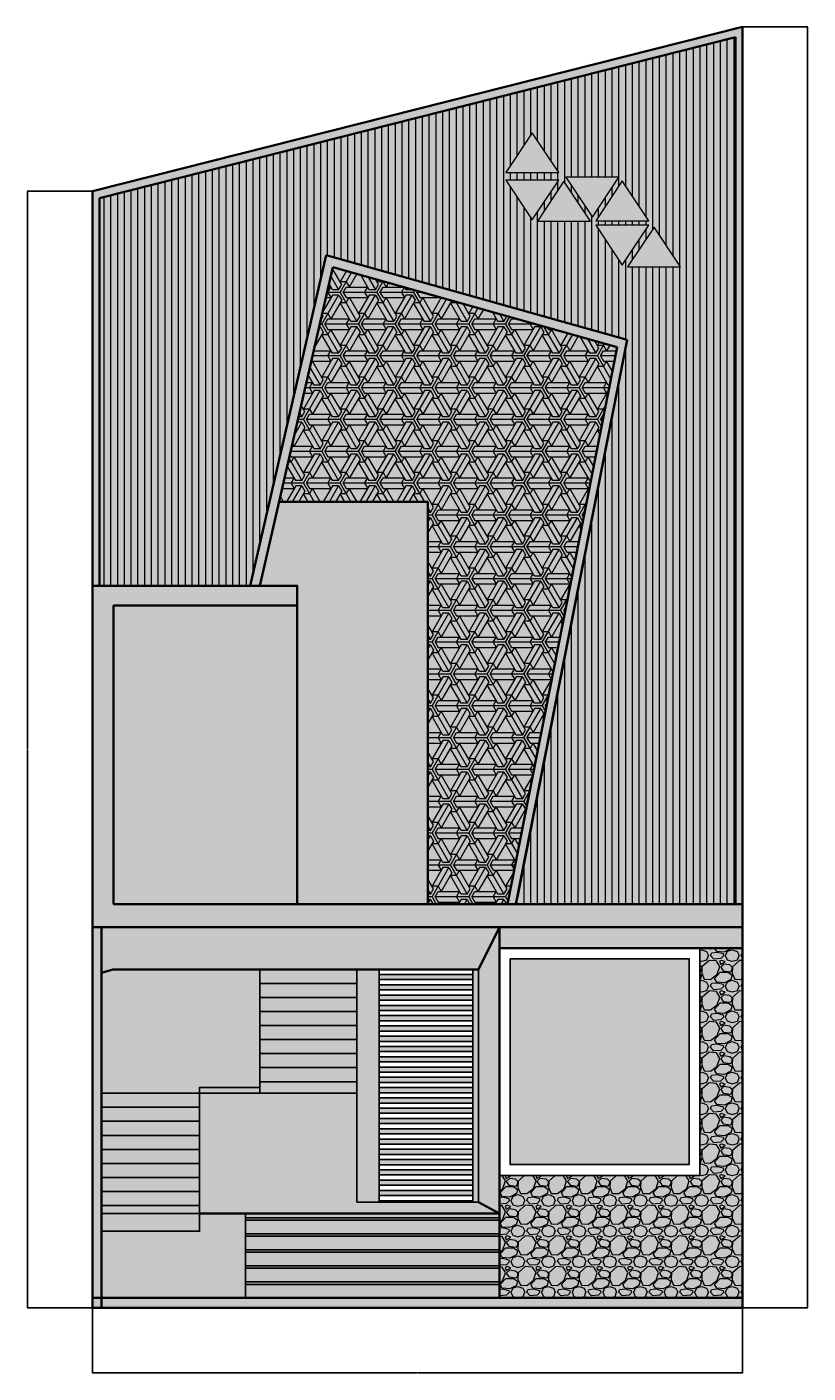
# Model space of a CAD drawing. Units: feet. Extents: x 2373 to 3800, y 799 to 1842.
# Tile 1 of 4: x 2373 to 2950, y 799 to 1794. Entities that reach past the tile are written whole.
import ezdxf

# ---------------------------------------------------------------- set-up
doc = ezdxf.new("R2010")
doc.units = ezdxf.units.FT
for name, color, linetype, lineweight in [('A-ANNO-DIMS', 2, 'Continuous', 18), ('A-DOOR', 4, 'Continuous', 25), ('A-ELEV', 7, 'Continuous', 35), ('A-ELEV-PATT', 8, 'Continuous', 13), ('A-FLOR-STRS', 3, 'Continuous', 25), ('A-GLAZ', 4, 'Continuous', 25), ('E-LITE', 2, 'Continuous', 18)]:
    doc.layers.add(name, color=color, linetype=linetype, lineweight=lineweight)
doc.styles.get("Standard").update_dxf_attribs({"font": 'arial.ttf'})
doc.dimstyles.get("Standard").update_dxf_attribs({"dimtxt": 0.18, "dimasz": 0.18, "dimexe": 0.18, "dimexo": 0.0625, "dimgap": 0.09, "dimtad": 0, "dimtih": 1, "dimtoh": 1, "dimdec": 1, "dimzin": 0, "dimdsep": 46, "dimlunit": 3, "dimtxsty": 'Standard', "dimcen": 0.09, "dimadec": 0, "dimazin": 0, "dimtfac": 1, "dimtdec": 1, "dimtofl": 0, "dimtmove": 0, "dimatfit": 3, "dimfxl": 1, "dimtolj": 1, "dimtzin": 0, "dimarcsym": 0})

# ---------------------------------------------------------------- blocks, each defined once
blk = doc.blocks.new('LIGHT-TRIANGLE')
blk.add_lwpolyline([(2765.64, 1685.95), (2746.09, 1715.45), (2726.54, 1685.95)], close=True)
blk = doc.blocks.new('*D4')
at = {"layer": 'A-ANNO-DIMS', "color": 0, "lineweight": -2, "transparency": 16777216}
for p, q in [((2421.33, 847.59), (2421.33, 799.47)), ((2901.33, 847.59), (2901.33, 799.47)), ((2421.51, 799.65), (2661.04, 799.65)), ((2901.15, 799.65), (2661.62, 799.65))]:
    blk.add_line(p, q, dxfattribs=at)
at = {"layer": 'A-ANNO-DIMS', "color": 0, "transparency": 16777216}
for points in [[(2421.51, 799.68), (2421.51, 799.62), (2421.33, 799.65)], [(2901.15, 799.68), (2901.15, 799.62), (2901.33, 799.65)]]:
    blk.add_solid(points, dxfattribs=at)
at = {"layer": 'Defpoints', "color": 0, "transparency": 16777216}
for p in [(2421.33, 847.65), (2901.33, 847.65), (2901.33, 799.65)]:
    blk.add_point(p, dxfattribs=at)
at = {"layer": 'A-ANNO-DIMS', "color": 0, "transparency": 16777216, "insert": (2661.33, 799.65), "char_height": 0.18, "attachment_point": 5}
blk.add_mtext('\\A1;480', dxfattribs=at)
blk = doc.blocks.new('*D5')
at = {"layer": 'A-ANNO-DIMS', "color": 0, "lineweight": -2, "transparency": 16777216}
for p, q in [((2901.39, 1793.54), (2949.51, 1793.54)), ((2949.33, 1793.36), (2949.33, 1320.78)), ((2949.33, 847.83), (2949.33, 1320.41)), ((2901.39, 847.65), (2949.51, 847.65))]:
    blk.add_line(p, q, dxfattribs=at)
at = {"layer": 'A-ANNO-DIMS', "color": 0, "transparency": 16777216}
for points in [[(2949.3, 1793.36), (2949.36, 1793.36), (2949.33, 1793.54)], [(2949.3, 847.83), (2949.36, 847.83), (2949.33, 847.65)]]:
    blk.add_solid(points, dxfattribs=at)
at = {"layer": 'Defpoints', "color": 0, "transparency": 16777216}
for p in [(2901.33, 1793.54), (2949.33, 1793.54), (2901.33, 847.65)]:
    blk.add_point(p, dxfattribs=at)
at = {"layer": 'A-ANNO-DIMS', "color": 0, "transparency": 16777216, "insert": (2949.33, 1320.6), "char_height": 0.18, "attachment_point": 5}
blk.add_mtext('\\A1;945.9', dxfattribs=at)
blk = doc.blocks.new('*D6')
at = {"layer": 'A-ANNO-DIMS', "color": 0, "lineweight": -2, "transparency": 16777216}
for p, q in [((2421.27, 1672.17), (2373.15, 1672.17)), ((2373.33, 1671.99), (2373.33, 1260.09)), ((2373.33, 847.83), (2373.33, 1259.73)), ((2421.27, 847.65), (2373.15, 847.65))]:
    blk.add_line(p, q, dxfattribs=at)
at = {"layer": 'A-ANNO-DIMS', "color": 0, "transparency": 16777216}
for points in [[(2373.3, 1671.99), (2373.36, 1671.99), (2373.33, 1672.17)], [(2373.3, 847.83), (2373.36, 847.83), (2373.33, 847.65)]]:
    blk.add_solid(points, dxfattribs=at)
at = {"layer": 'Defpoints', "color": 0, "transparency": 16777216}
for p in [(2373.33, 1672.17), (2421.33, 1672.17), (2421.33, 847.65)]:
    blk.add_point(p, dxfattribs=at)
at = {"layer": 'A-ANNO-DIMS', "color": 0, "transparency": 16777216, "insert": (2373.33, 1259.91), "char_height": 0.18, "attachment_point": 5}
blk.add_mtext('\\A1;824.5', dxfattribs=at)

msp = doc.modelspace()

# ---------------------------------------------------------------- hatches: boundary and pattern name
at = {"layer": 'A-ELEV-PATT'}
h = msp.add_hatch(color=256, dxfattribs=at)
h.dxf.hatch_style = 1
h.paths.add_polyline_path([(2426.4685, 1667.1821), (2896.1905, 1785.9513), (2896.1905, 1145.7869), (2901.3295, 1145.7869), (2901.3295, 1793.536), (2421.3295, 1672.168), (2421.3295, 1380.85), (2426.4685, 1380.85)])
h = msp.add_hatch(color=256, dxfattribs=at)
h.dxf.hatch_style = 1
h.paths.add_polyline_path([(2593.8631, 1624.879), (2816.0008, 1562.4189), (2734.0244, 1145.7869), (2896.1905, 1145.7869), (2896.1905, 1785.9513), (2426.4685, 1667.1821), (2426.4685, 1380.85), (2537.8601, 1380.85)])
h.paths.add_polyline_path([(2726.5383, 1680.4979), (2765.6367, 1680.4979), (2746.0875, 1650.9943)], flags=16)
h.paths.add_polyline_path([(2726.5383, 1685.9478), (2746.0875, 1715.4514), (2765.6367, 1685.9478)], flags=16)
h.paths.add_polyline_path([(2749.8119, 1650.1162), (2769.3612, 1679.6197), (2788.9104, 1650.1162)], flags=16)
h.paths.add_polyline_path([(2770.8786, 1682.5998), (2809.977, 1682.5998), (2790.4278, 1653.0963)], flags=16)
h.paths.add_polyline_path([(2792.9281, 1647.0854), (2832.0266, 1647.0854), (2812.4773, 1617.5819)], flags=16)
h.paths.add_polyline_path([(2792.956, 1650.2964), (2812.5053, 1679.7999), (2832.0545, 1650.2964)], flags=16)
h.paths.add_polyline_path([(2816.44, 1616.2701), (2835.9892, 1645.7737), (2855.5384, 1616.2701)], flags=16)
h = msp.add_hatch(dxfattribs=at)
h.set_pattern_fill('_USER', color=256, scale=5, angle=90, style=0, pattern_type=0)
h.set_pattern_definition([(90, (0, 0), (-5, 3e-16), [])])
h.paths.add_polyline_path([(2593.8631, 1624.879), (2816.0008, 1562.4189), (2735.0715, 1151.1084), (2734.0244, 1145.7869), (2896.1905, 1145.7869), (2896.1905, 1785.9513), (2426.4685, 1667.1821), (2426.4685, 1380.85), (2537.8601, 1380.85)])
h.paths.add_polyline_path([(2726.5383, 1680.4979), (2765.6367, 1680.4979), (2746.0875, 1650.9943)], flags=16)
h.paths.add_polyline_path([(2726.5383, 1685.9478), (2746.0875, 1715.4514), (2765.6367, 1685.9478)], flags=16)
h.paths.add_polyline_path([(2749.8119, 1650.1162), (2769.3612, 1679.6197), (2788.9104, 1650.1162)], flags=16)
h.paths.add_polyline_path([(2770.8786, 1682.5998), (2809.977, 1682.5998), (2790.4278, 1653.0963)], flags=16)
h.paths.add_polyline_path([(2792.9281, 1647.0854), (2832.0266, 1647.0854), (2812.4773, 1617.5819)], flags=16)
h.paths.add_polyline_path([(2792.956, 1650.2964), (2812.5053, 1679.7999), (2832.0545, 1650.2964)], flags=16)
h.paths.add_polyline_path([(2816.44, 1616.2701), (2835.9892, 1645.7737), (2855.5384, 1616.2701)], flags=16)
h = msp.add_hatch(color=256, dxfattribs=at)
h.dxf.hatch_style = 1
h.paths.add_polyline_path([(2746.0875, 1715.4514), (2726.5383, 1685.9478), (2765.6367, 1685.9478)])
h.paths.add_polyline_path([(2765.6367, 1680.4979), (2726.5383, 1680.4979), (2746.0875, 1650.9943)])
h.paths.add_polyline_path([(2769.3612, 1679.6197), (2749.8119, 1650.1162), (2788.9104, 1650.1162)])
h.paths.add_polyline_path([(2809.977, 1682.5998), (2770.8786, 1682.5998), (2790.4278, 1653.0963)])
h.paths.add_polyline_path([(2812.5053, 1679.7999), (2792.956, 1650.2964), (2832.0545, 1650.2964)])
h.paths.add_polyline_path([(2832.0266, 1647.0854), (2792.9281, 1647.0854), (2812.4773, 1617.5819)])
h.paths.add_polyline_path([(2835.9892, 1645.7737), (2816.44, 1616.2701), (2855.5384, 1616.2701)])
h.paths.add_polyline_path([(2901.3295, 1145.7869), (2436.8307, 1145.7869), (2436.8307, 1366.1757), (2572.5359, 1366.1757), (2572.5359, 1380.85), (2537.8601, 1380.85), (2421.3295, 1380.85), (2421.3295, 1366.1757), (2421.3295, 1128.6662), (2901.3295, 1128.6662)])
h = msp.add_hatch(color=256, dxfattribs=at)
h.dxf.hatch_style = 1
h.paths.add_polyline_path([(2598.9204, 1616.114), (2808.8118, 1557.0974), (2727.8825, 1145.7869), (2734.0244, 1145.7869), (2816.0008, 1562.4189), (2593.8631, 1624.879), (2537.8601, 1380.85), (2544.9289, 1380.85)])
h.paths.add_polyline_path([(2427.9464, 1128.6662), (2421.3295, 1128.6662), (2421.3295, 847.6543), (2427.9464, 847.6543)])
h.paths.add_polyline_path([(2500.519, 917.36), (2427.9464, 917.36), (2427.9464, 904.1787), (2500.519, 904.1787)])
h.paths.add_polyline_path([(2721.7769, 864.9874), (2534.3062, 864.9874), (2534.3062, 854.9626), (2721.7769, 854.9626)])
h.paths.add_polyline_path([(2721.7769, 876.8247), (2534.3062, 876.8247), (2534.3062, 866.7999), (2721.7769, 866.7999)])
h.paths.add_polyline_path([(2721.7769, 888.662), (2534.3062, 888.662), (2534.3062, 878.6372), (2721.7769, 878.6372)])
h.paths.add_polyline_path([(2721.7769, 900.4994), (2534.3062, 900.4994), (2534.3062, 890.4745), (2721.7769, 890.4745)])
h.paths.add_polyline_path([(2721.7769, 912.3367), (2534.3062, 912.3367), (2534.3062, 902.3118), (2721.7769, 902.3118)])
h.paths.add_polyline_path([(2721.7769, 917.36), (2534.3062, 917.36), (2534.3062, 914.1491), (2721.7769, 914.1491)])
h.paths.add_polyline_path([(2901.3295, 854.9626), (2721.7769, 854.9626), (2534.3062, 854.9626), (2427.9464, 854.9626), (2427.9464, 847.6543), (2901.3295, 847.6543)])
h = msp.add_hatch(color=256, dxfattribs=at)
h.dxf.hatch_style = 1
h.paths.add_polyline_path([(2808.8118, 1557.0974), (2598.9204, 1616.114), (2559.1388, 1442.7685), (2669.0801, 1442.7685), (2669.0801, 1145.7869), (2727.8825, 1145.7869)])
h = msp.add_hatch(dxfattribs=at)
h.set_pattern_fill('ESCHER', color=256, scale=0.89)
h.paths.add_polyline_path([(2808.8118, 1557.0974), (2598.9204, 1616.114), (2559.1388, 1442.7685), (2669.0801, 1442.7685), (2669.0801, 1145.7869), (2727.8825, 1145.7869)])
h = msp.add_hatch(color=256, dxfattribs=at)
h.dxf.hatch_style = 1
h.paths.add_polyline_path([(2669.0801, 1442.7685), (2559.1388, 1442.7685), (2544.9289, 1380.85), (2572.5359, 1380.85), (2572.5359, 1145.7869), (2669.0801, 1145.7869)])
h.paths.add_polyline_path([(2702.0866, 1093.7911), (2632.9975, 1093.7911), (2632.9975, 1089.9953), (2702.0866, 1089.9953)])
h.paths.add_polyline_path([(2702.0866, 1086.1996), (2632.9975, 1086.1996), (2632.9975, 1082.4038), (2702.0866, 1082.4038)])
h.paths.add_polyline_path([(2702.0866, 1078.6081), (2632.9975, 1078.6081), (2632.9975, 1074.8123), (2702.0866, 1074.8123)])
h.paths.add_polyline_path([(2702.0866, 1071.0166), (2632.9975, 1071.0166), (2632.9975, 1067.2208), (2702.0866, 1067.2208)])
h = msp.add_hatch(color=256, dxfattribs=at)
h.paths.add_polyline_path([(2572.5359, 1366.1757), (2436.8307, 1366.1757), (2436.8307, 1145.7869), (2572.5359, 1145.7869)])
h.paths.add_polyline_path([(2861.7756, 1105.4077), (2729.7295, 1105.4077), (2729.7295, 953.4176), (2861.7756, 953.4176)])
h = msp.add_hatch(color=256, dxfattribs=at)
h.dxf.hatch_style = 1
h.paths.add_polyline_path([(2721.7769, 1128.6662), (2427.9464, 1128.6662), (2427.9464, 1095.1425), (2436.5092, 1097.5869), (2706.3668, 1097.5869)])
h.paths.add_polyline_path([(2901.3295, 1113.3603), (2869.7282, 1113.3603), (2869.7282, 945.465), (2721.7769, 945.465), (2721.7769, 854.9626), (2901.3295, 854.9626)])
h = msp.add_hatch(color=256, dxfattribs=at)
h.dxf.hatch_style = 1
h.paths.add_polyline_path([(2632.9975, 1097.5869), (2616.4601, 1097.5869), (2616.4601, 1006.1175), (2616.4601, 925.687), (2632.9975, 925.687)])
h.paths.add_polyline_path([(2706.3668, 1097.5869), (2702.0866, 1097.5869), (2702.0866, 925.687), (2706.3668, 925.687)])
h.paths.add_polyline_path([(2721.7769, 1113.3603), (2721.7769, 1128.6662), (2706.3668, 1097.5869), (2706.3668, 925.687), (2721.7769, 917.36)])
h = msp.add_hatch(color=256, dxfattribs=at)
h.dxf.hatch_style = 1
h.paths.add_polyline_path([(2901.3295, 1128.6662), (2721.7769, 1128.6662), (2721.7769, 1113.3603), (2869.7282, 1113.3603), (2901.3295, 1113.3603)])
h = msp.add_hatch(dxfattribs=at)
h.set_pattern_fill('GRAVEL', color=256, scale=0.89)
h.paths.add_polyline_path([(2901.3295, 1113.3603), (2869.7282, 1113.3603), (2869.7282, 945.465), (2721.7769, 945.465), (2721.7769, 854.9626), (2901.3295, 854.9626)])
h = msp.add_hatch(color=256, dxfattribs=at)
h.dxf.hatch_style = 1
h.paths.add_polyline_path([(2616.4601, 1097.5869), (2544.8251, 1097.5869), (2544.8251, 1087.2185), (2616.4601, 1087.2185)])
h.paths.add_polyline_path([(2616.4601, 1087.2185), (2544.8251, 1087.2185), (2544.8251, 1076.8502), (2616.4601, 1076.8502)])
h.paths.add_polyline_path([(2616.4601, 1076.8502), (2544.8251, 1076.8502), (2544.8251, 1066.4819), (2616.4601, 1066.4819)])
h.paths.add_polyline_path([(2616.4601, 1056.1136), (2544.8251, 1056.1136), (2544.8251, 1045.7452), (2616.4601, 1045.7452)])
h.paths.add_polyline_path([(2616.4601, 1066.4819), (2544.8251, 1066.4819), (2544.8251, 1056.1136), (2616.4601, 1056.1136)])
h.paths.add_polyline_path([(2616.4601, 1045.7452), (2544.8251, 1045.7452), (2544.8251, 1035.3769), (2616.4601, 1035.3769)])
h.paths.add_polyline_path([(2616.4601, 1035.3769), (2544.8251, 1035.3769), (2544.8251, 1025.0086), (2616.4601, 1025.0086)])
h.paths.add_polyline_path([(2616.4601, 1025.0086), (2544.8251, 1025.0086), (2544.8251, 1014.6403), (2616.4601, 1014.6403)])
h.paths.add_polyline_path([(2616.4601, 1014.6403), (2544.8251, 1014.6403), (2544.8251, 1006.1175), (2616.4601, 1006.1175)])
h.paths.add_polyline_path([(2544.8251, 1056.1136), (2544.8251, 1066.4819), (2544.8251, 1076.8502), (2544.8251, 1087.2185), (2544.8251, 1097.5869), (2436.5092, 1097.5869), (2427.9464, 1095.1425), (2427.9464, 1006.1175), (2500.519, 1006.1175), (2500.519, 1010.4128), (2544.8251, 1010.4128), (2544.8251, 1014.6403), (2544.8251, 1025.0086), (2544.8251, 1035.3769), (2544.8251, 1045.7452)])
h = msp.add_hatch(color=256, dxfattribs=at)
h.dxf.hatch_style = 1
h.paths.add_polyline_path([(2702.0866, 1063.4251), (2632.9975, 1063.4251), (2632.9975, 1059.6293), (2702.0866, 1059.6293)])
h = msp.add_hatch(color=256, dxfattribs=at)
h.dxf.hatch_style = 1
h.paths.add_polyline_path([(2702.0866, 1055.8336), (2632.9975, 1055.8336), (2632.9975, 1052.0378), (2702.0866, 1052.0378)])
h = msp.add_hatch(color=256, dxfattribs=at)
h.dxf.hatch_style = 1
h.paths.add_polyline_path([(2702.0866, 1048.2421), (2632.9975, 1048.2421), (2632.9975, 1044.4463), (2702.0866, 1044.4463)])
h = msp.add_hatch(color=256, dxfattribs=at)
h.dxf.hatch_style = 1
h.paths.add_polyline_path([(2702.0866, 1040.6506), (2632.9975, 1040.6506), (2632.9975, 1036.8548), (2702.0866, 1036.8548)])
h = msp.add_hatch(color=256, dxfattribs=at)
h.dxf.hatch_style = 1
h.paths.add_polyline_path([(2702.0866, 1033.059), (2632.9975, 1033.059), (2632.9975, 1029.2633), (2702.0866, 1029.2633)])
h = msp.add_hatch(color=256, dxfattribs=at)
h.dxf.hatch_style = 1
h.paths.add_polyline_path([(2702.0866, 1025.4675), (2632.9975, 1025.4675), (2632.9975, 1021.6718), (2702.0866, 1021.6718)])
h = msp.add_hatch(color=256, dxfattribs=at)
h.dxf.hatch_style = 1
h.paths.add_polyline_path([(2702.0866, 1017.876), (2632.9975, 1017.876), (2632.9975, 1014.0803), (2702.0866, 1014.0803)])
h = msp.add_hatch(color=256, dxfattribs=at)
h.dxf.hatch_style = 1
h.paths.add_polyline_path([(2616.4601, 1006.1175), (2544.8251, 1006.1175), (2500.519, 1006.1175), (2500.519, 917.36), (2721.7769, 917.36), (2706.3668, 925.687), (2616.4601, 925.687)])
h.paths.add_polyline_path([(2500.519, 995.7492), (2427.9464, 995.7492), (2427.9464, 985.3808), (2500.519, 985.3808)])
h.paths.add_polyline_path([(2500.519, 1006.1175), (2427.9464, 1006.1175), (2427.9464, 995.7492), (2500.519, 995.7492)])
h.paths.add_polyline_path([(2500.519, 985.3808), (2427.9464, 985.3808), (2427.9464, 975.0125), (2500.519, 975.0125)])
h.paths.add_polyline_path([(2500.519, 975.0125), (2427.9464, 975.0125), (2427.9464, 964.6442), (2500.519, 964.6442)])
h.paths.add_polyline_path([(2500.519, 964.6442), (2427.9464, 964.6442), (2427.9464, 954.2759), (2500.519, 954.2759)])
h.paths.add_polyline_path([(2500.519, 954.2759), (2427.9464, 954.2759), (2427.9464, 943.9075), (2500.519, 943.9075)])
h.paths.add_polyline_path([(2500.519, 943.9075), (2427.9464, 943.9075), (2427.9464, 933.5392), (2500.519, 933.5392)])
h.paths.add_polyline_path([(2500.519, 933.5392), (2427.9464, 933.5392), (2427.9464, 923.1709), (2500.519, 923.1709)])
h.paths.add_polyline_path([(2500.519, 923.1709), (2427.9464, 923.1709), (2427.9464, 917.36), (2500.519, 917.36)])
h.paths.add_polyline_path([(2544.8251, 1010.4128), (2500.519, 1010.4128), (2500.519, 1006.1175), (2544.8251, 1006.1175)])
h.paths.add_polyline_path([(2721.7769, 878.6372), (2534.3062, 878.6372), (2534.3062, 876.8247), (2721.7769, 876.8247)])
h.paths.add_polyline_path([(2721.7769, 866.7999), (2534.3062, 866.7999), (2534.3062, 864.9874), (2721.7769, 864.9874)])
h.paths.add_polyline_path([(2721.7769, 890.4745), (2534.3062, 890.4745), (2534.3062, 888.662), (2721.7769, 888.662)])
h.paths.add_polyline_path([(2721.7769, 902.3118), (2534.3062, 902.3118), (2534.3062, 900.4994), (2721.7769, 900.4994)])
h.paths.add_polyline_path([(2721.7769, 914.1491), (2534.3062, 914.1491), (2534.3062, 912.3367), (2721.7769, 912.3367)])
h = msp.add_hatch(color=256, dxfattribs=at)
h.dxf.hatch_style = 1
h.paths.add_polyline_path([(2702.0866, 1010.2845), (2632.9975, 1010.2845), (2632.9975, 1006.4888), (2702.0866, 1006.4888)])
h = msp.add_hatch(color=256, dxfattribs=at)
h.dxf.hatch_style = 1
h.paths.add_polyline_path([(2702.0866, 1002.693), (2632.9975, 1002.693), (2632.9975, 998.8973), (2702.0866, 998.8973)])
h = msp.add_hatch(color=256, dxfattribs=at)
h.dxf.hatch_style = 1
h.paths.add_polyline_path([(2702.0866, 995.1015), (2632.9975, 995.1015), (2632.9975, 991.3058), (2702.0866, 991.3058)])
h = msp.add_hatch(color=256, dxfattribs=at)
h.dxf.hatch_style = 1
h.paths.add_polyline_path([(2702.0866, 987.51), (2632.9975, 987.51), (2632.9975, 983.7143), (2702.0866, 983.7143)])
h = msp.add_hatch(color=256, dxfattribs=at)
h.dxf.hatch_style = 1
h.paths.add_polyline_path([(2702.0866, 979.9185), (2632.9975, 979.9185), (2632.9975, 976.1228), (2702.0866, 976.1228)])
h = msp.add_hatch(color=256, dxfattribs=at)
h.dxf.hatch_style = 1
h.paths.add_polyline_path([(2702.0866, 972.327), (2632.9975, 972.327), (2632.9975, 968.5312), (2702.0866, 968.5312)])
h = msp.add_hatch(color=256, dxfattribs=at)
h.dxf.hatch_style = 1
h.paths.add_polyline_path([(2702.0866, 964.7355), (2632.9975, 964.7355), (2632.9975, 960.9397), (2702.0866, 960.9397)])
h = msp.add_hatch(color=256, dxfattribs=at)
h.dxf.hatch_style = 1
h.paths.add_polyline_path([(2702.0866, 957.144), (2632.9975, 957.144), (2632.9975, 953.3482), (2702.0866, 953.3482)])
h = msp.add_hatch(color=256, dxfattribs=at)
h.dxf.hatch_style = 1
h.paths.add_polyline_path([(2702.0866, 949.5525), (2632.9975, 949.5525), (2632.9975, 945.7567), (2702.0866, 945.7567)])
h = msp.add_hatch(color=256, dxfattribs=at)
h.dxf.hatch_style = 1
h.paths.add_polyline_path([(2702.0866, 941.961), (2632.9975, 941.961), (2632.9975, 938.1652), (2702.0866, 938.1652)])
h = msp.add_hatch(color=256, dxfattribs=at)
h.dxf.hatch_style = 1
h.paths.add_polyline_path([(2702.0866, 934.3695), (2632.9975, 934.3695), (2632.9975, 930.5737), (2702.0866, 930.5737)])
h = msp.add_hatch(color=256, dxfattribs=at)
h.dxf.hatch_style = 1
h.paths.add_polyline_path([(2702.0866, 926.778), (2632.9975, 926.778), (2632.9975, 925.687), (2702.0866, 925.687)])
msp.add_hatch(color=256, dxfattribs=at).paths.add_polyline_path([(2534.3062, 917.36), (2500.519, 917.36), (2500.519, 904.1787), (2427.9464, 904.1787), (2427.9464, 854.9626), (2534.3062, 854.9626)])

# ---------------------------------------------------------------- linework, layer by layer
at = {"layer": 'A-DOOR'}
for p, q in [((2616.4601, 925.687), (2616.4601, 1097.5869)), ((2616.4601, 925.687), (2616.4601, 1097.5869)), ((2632.9975, 1093.7911), (2702.0866, 1093.7911)), ((2632.9975, 1093.7911), (2702.0866, 1093.7911)), ((2706.3668, 1097.5869), (2706.3668, 925.687)), ((2706.3668, 1097.5869), (2706.3668, 925.687)), ((2632.9975, 1089.9953), (2702.0866, 1089.9953)), ((2632.9975, 1089.9953), (2702.0866, 1089.9953)), ((2632.9975, 1086.1996), (2702.0866, 1086.1996)), ((2632.9975, 1086.1996), (2702.0866, 1086.1996)), ((2632.9975, 1082.4038), (2702.0866, 1082.4038)), ((2632.9975, 1082.4038), (2702.0866, 1082.4038)), ((2632.9975, 1078.6081), (2702.0866, 1078.6081)), ((2632.9975, 1078.6081), (2702.0866, 1078.6081)), ((2632.9975, 1074.8123), (2702.0866, 1074.8123)), ((2632.9975, 1074.8123), (2702.0866, 1074.8123)), ((2632.9975, 1071.0166), (2702.0866, 1071.0166)), ((2632.9975, 1071.0166), (2702.0866, 1071.0166)), ((2632.9975, 1067.2208), (2702.0866, 1067.2208)), ((2632.9975, 1067.2208), (2702.0866, 1067.2208)), ((2632.9975, 1063.4251), (2702.0866, 1063.4251)), ((2632.9975, 1063.4251), (2702.0866, 1063.4251)), ((2632.9975, 1059.6293), (2702.0866, 1059.6293)), ((2632.9975, 1059.6293), (2702.0866, 1059.6293)), ((2632.9975, 1055.8336), (2702.0866, 1055.8336)), ((2632.9975, 1055.8336), (2702.0866, 1055.8336)), ((2632.9975, 1052.0378), (2702.0866, 1052.0378)), ((2632.9975, 1052.0378), (2702.0866, 1052.0378)), ((2632.9975, 1048.2421), (2702.0866, 1048.2421)), ((2632.9975, 1048.2421), (2702.0866, 1048.2421)), ((2632.9975, 1044.4463), (2702.0866, 1044.4463)), ((2632.9975, 1044.4463), (2702.0866, 1044.4463)), ((2632.9975, 1040.6506), (2702.0866, 1040.6506)), ((2632.9975, 1040.6506), (2702.0866, 1040.6506)), ((2632.9975, 1036.8548), (2702.0866, 1036.8548)), ((2632.9975, 1036.8548), (2702.0866, 1036.8548)), ((2632.9975, 1033.059), (2702.0866, 1033.059)), ((2632.9975, 1033.059), (2702.0866, 1033.059)), ((2632.9975, 1029.2633), (2702.0866, 1029.2633)), ((2632.9975, 1029.2633), (2702.0866, 1029.2633)), ((2632.9975, 1025.4675), (2702.0866, 1025.4675)), ((2632.9975, 1025.4675), (2702.0866, 1025.4675)), ((2632.9975, 1021.6718), (2702.0866, 1021.6718)), ((2632.9975, 1021.6718), (2702.0866, 1021.6718)), ((2632.9975, 1017.876), (2702.0866, 1017.876)), ((2632.9975, 1017.876), (2702.0866, 1017.876)), ((2632.9975, 1014.0803), (2702.0866, 1014.0803)), ((2632.9975, 1014.0803), (2702.0866, 1014.0803)), ((2632.9975, 1010.2845), (2702.0866, 1010.2845)), ((2632.9975, 1010.2845), (2702.0866, 1010.2845)), ((2632.9975, 1006.4888), (2702.0866, 1006.4888)), ((2632.9975, 1006.4888), (2702.0866, 1006.4888)), ((2632.9975, 1002.693), (2702.0866, 1002.693)), ((2632.9975, 1002.693), (2702.0866, 1002.693)), ((2632.9975, 998.8973), (2702.0866, 998.8973)), ((2632.9975, 998.8973), (2702.0866, 998.8973)), ((2632.9975, 995.1015), (2702.0866, 995.1015)), ((2632.9975, 995.1015), (2702.0866, 995.1015)), ((2632.9975, 991.3058), (2702.0866, 991.3058)), ((2632.9975, 991.3058), (2702.0866, 991.3058)), ((2632.9975, 987.51), (2702.0866, 987.51)), ((2632.9975, 987.51), (2702.0866, 987.51)), ((2632.9975, 983.7143), (2702.0866, 983.7143)), ((2632.9975, 983.7143), (2702.0866, 983.7143)), ((2632.9975, 979.9185), (2702.0866, 979.9185)), ((2632.9975, 979.9185), (2702.0866, 979.9185)), ((2632.9975, 976.1228), (2702.0866, 976.1228)), ((2632.9975, 976.1228), (2702.0866, 976.1228)), ((2632.9975, 972.327), (2702.0866, 972.327)), ((2632.9975, 972.327), (2702.0866, 972.327)), ((2632.9975, 968.5312), (2702.0866, 968.5312)), ((2632.9975, 968.5312), (2702.0866, 968.5312)), ((2632.9975, 964.7355), (2702.0866, 964.7355)), ((2632.9975, 964.7355), (2702.0866, 964.7355)), ((2632.9975, 960.9397), (2702.0866, 960.9397)), ((2632.9975, 960.9397), (2702.0866, 960.9397)), ((2632.9975, 957.144), (2702.0866, 957.144)), ((2632.9975, 957.144), (2702.0866, 957.144)), ((2632.9975, 953.3482), (2702.0866, 953.3482)), ((2632.9975, 953.3482), (2702.0866, 953.3482)), ((2632.9975, 949.5525), (2702.0866, 949.5525)), ((2632.9975, 949.5525), (2702.0866, 949.5525)), ((2632.9975, 945.7567), (2702.0866, 945.7567)), ((2632.9975, 945.7567), (2702.0866, 945.7567)), ((2632.9975, 941.961), (2702.0866, 941.961)), ((2632.9975, 941.961), (2702.0866, 941.961)), ((2632.9975, 938.1652), (2702.0866, 938.1652)), ((2632.9975, 938.1652), (2702.0866, 938.1652)), ((2706.3668, 925.687), (2616.4601, 925.687)), ((2706.3668, 925.687), (2616.4601, 925.687)), ((2632.9975, 934.3695), (2702.0866, 934.3695)), ((2632.9975, 934.3695), (2702.0866, 934.3695)), ((2632.9975, 930.5737), (2702.0866, 930.5737)), ((2632.9975, 930.5737), (2702.0866, 930.5737)), ((2632.9975, 926.778), (2702.0866, 926.778)), ((2632.9975, 926.778), (2702.0866, 926.778))]:
    msp.add_line(p, q, dxfattribs=at)
msp.add_lwpolyline([(2702.0866, 925.687), (2632.9975, 925.687), (2632.9975, 1097.5869), (2702.0866, 1097.5869)], close=True, dxfattribs=at)
msp.add_lwpolyline([(2702.0866, 925.687), (2632.9975, 925.687), (2632.9975, 1097.5869), (2702.0866, 1097.5869)], close=True, dxfattribs=at)
at = {"layer": 'A-ELEV'}
for p, q in [((2421.3295, 1672.168), (2901.3295, 1793.536)), ((2421.3295, 1672.168), (2901.3295, 1793.536)), ((2901.3295, 847.6543), (2901.3295, 1793.536)), ((2901.3295, 847.6543), (2901.3295, 1793.536)), ((2426.4685, 1667.1821), (2896.1905, 1785.9513)), ((2426.4685, 1667.1821), (2896.1905, 1785.9513)), ((2896.1905, 1785.9513), (2896.1905, 1145.7869)), ((2896.1905, 1785.9513), (2896.1905, 1145.7869)), ((2421.3295, 847.6543), (2421.3295, 1672.168)), ((2421.3295, 847.6543), (2421.3295, 1672.168)), ((2426.4685, 1667.1821), (2426.4685, 1380.85)), ((2426.4685, 1667.1821), (2426.4685, 1380.85)), ((2593.8631, 1624.879), (2537.8601, 1380.85)), ((2593.8631, 1624.879), (2537.8601, 1380.85)), ((2593.8631, 1624.879), (2816.0008, 1562.4189)), ((2593.8631, 1624.879), (2816.0008, 1562.4189)), ((2598.9204, 1616.114), (2544.9289, 1380.85)), ((2598.9204, 1616.114), (2544.9289, 1380.85)), ((2598.9204, 1616.114), (2808.8118, 1557.0974)), ((2598.9204, 1616.114), (2808.8118, 1557.0974)), ((2734.0244, 1145.7869), (2816.0008, 1562.4189)), ((2735.0715, 1151.1084), (2816.0008, 1562.4189)), ((2727.8825, 1145.7869), (2808.8118, 1557.0974)), ((2727.8825, 1145.7869), (2808.8118, 1557.0974)), ((2706.3668, 1097.5869), (2721.7769, 1128.6662)), ((2706.3668, 1097.5869), (2721.7769, 1128.6662)), ((2721.7769, 1113.3603), (2721.7769, 1128.6662)), ((2721.7769, 1113.3603), (2721.7769, 1128.6662)), ((2436.5092, 1097.5869), (2427.9464, 1095.1425)), ((2436.5092, 1097.5869), (2427.9464, 1095.1425)), ((2706.3668, 1097.5869), (2436.5092, 1097.5869)), ((2706.3668, 1097.5869), (2436.5092, 1097.5869)), ((2706.3668, 925.687), (2721.7769, 917.36)), ((2706.3668, 925.687), (2721.7769, 917.36)), ((2721.7769, 917.36), (2500.519, 917.36)), ((2721.7769, 917.36), (2500.519, 917.36)), ((2421.3295, 847.6543), (2901.3295, 847.6543)), ((2421.3295, 847.6543), (2901.3295, 847.6543))]:
    msp.add_line(p, q, dxfattribs=at)
for points in [[(2559.1388, 1442.7685), (2669.0801, 1442.7685)], [(2559.1388, 1442.7685), (2669.0801, 1442.7685)], [(2669.0801, 1442.7685), (2669.0801, 1145.7869), (2572.5359, 1145.7869), (2572.5359, 1380.85)], [(2669.0801, 1442.7685), (2669.0801, 1145.7869), (2572.5359, 1145.7869), (2572.5359, 1380.85)], [(2421.3295, 1366.1757), (2421.3295, 1380.85)], [(2537.8601, 1380.85), (2421.3295, 1380.85), (2421.3295, 1128.6662), (2436.8307, 1128.6662)], [(2537.8601, 1380.85), (2421.3295, 1380.85), (2421.3295, 1128.6662), (2436.8307, 1128.6662)], [(2421.3295, 1366.1757), (2421.3295, 1380.85)], [(2537.8601, 1380.85), (2572.5359, 1380.85), (2572.5359, 1366.1757), (2436.8307, 1366.1757)], [(2537.8601, 1380.85), (2572.5359, 1380.85), (2572.5359, 1366.1757), (2436.8307, 1366.1757)], [(2436.8307, 1145.7869), (2436.8307, 1366.1757)], [(2436.8307, 1145.7869), (2436.8307, 1366.1757)], [(2421.3295, 1145.7869), (2421.3295, 1128.6662), (2901.3295, 1128.6662), (2901.3295, 1145.7869), (2436.8307, 1145.7869)], [(2421.3295, 1145.7869), (2421.3295, 1128.6662), (2901.3295, 1128.6662), (2901.3295, 1145.7869), (2436.8307, 1145.7869)]]:
    msp.add_lwpolyline(points, dxfattribs=at)
for points in [[(2421.3295, 1128.6662), (2427.9464, 1128.6662), (2427.9464, 847.6543), (2421.3295, 847.6543)], [(2421.3295, 1128.6662), (2427.9464, 1128.6662), (2427.9464, 847.6543), (2421.3295, 847.6543)], [(2901.3295, 854.9626), (2721.7769, 854.9626), (2721.7769, 1113.3603), (2901.3295, 1113.3603)], [(2901.3295, 854.9626), (2721.7769, 854.9626), (2721.7769, 1113.3603), (2901.3295, 1113.3603)], [(2421.3295, 847.6543), (2901.3295, 847.6543), (2901.3295, 854.9626), (2421.3295, 854.9626)], [(2421.3295, 847.6543), (2901.3295, 847.6543), (2901.3295, 854.9626), (2421.3295, 854.9626)]]:
    msp.add_lwpolyline(points, close=True, dxfattribs=at)
at = {"layer": 'A-FLOR-STRS'}
for p, q in [((2544.8251, 1087.2185), (2616.4601, 1087.2185)), ((2544.8251, 1087.2185), (2616.4601, 1087.2185)), ((2544.8251, 1076.8502), (2616.4601, 1076.8502)), ((2544.8251, 1076.8502), (2616.4601, 1076.8502)), ((2544.8251, 1066.4819), (2616.4601, 1066.4819)), ((2544.8251, 1066.4819), (2616.4601, 1066.4819)), ((2544.8251, 1056.1136), (2616.4601, 1056.1136)), ((2544.8251, 1056.1136), (2616.4601, 1056.1136)), ((2544.8251, 1045.7452), (2616.4601, 1045.7452)), ((2544.8251, 1045.7452), (2616.4601, 1045.7452)), ((2544.8251, 1035.3769), (2616.4601, 1035.3769)), ((2544.8251, 1035.3769), (2616.4601, 1035.3769)), ((2544.8251, 1025.0086), (2616.4601, 1025.0086)), ((2544.8251, 1025.0086), (2616.4601, 1025.0086)), ((2544.8251, 1014.6403), (2616.4601, 1014.6403)), ((2544.8251, 1014.6403), (2616.4601, 1014.6403)), ((2427.9464, 995.7492), (2500.519, 995.7492)), ((2427.9464, 995.7492), (2500.519, 995.7492)), ((2427.9464, 985.3808), (2500.519, 985.3808)), ((2427.9464, 985.3808), (2500.519, 985.3808)), ((2427.9464, 975.0125), (2500.519, 975.0125)), ((2427.9464, 975.0125), (2500.519, 975.0125)), ((2427.9464, 964.6442), (2500.519, 964.6442)), ((2427.9464, 964.6442), (2500.519, 964.6442)), ((2427.9464, 954.2759), (2500.519, 954.2759)), ((2427.9464, 954.2759), (2500.519, 954.2759)), ((2427.9464, 943.9075), (2500.519, 943.9075)), ((2427.9464, 943.9075), (2500.519, 943.9075)), ((2427.9464, 933.5392), (2500.519, 933.5392)), ((2427.9464, 933.5392), (2500.519, 933.5392)), ((2427.9464, 923.1709), (2500.519, 923.1709)), ((2427.9464, 923.1709), (2500.519, 923.1709)), ((2500.519, 917.36), (2427.9464, 917.36)), ((2500.519, 917.36), (2427.9464, 917.36)), ((2534.3062, 914.1491), (2721.7769, 914.1491)), ((2534.3062, 914.1491), (2721.7769, 914.1491)), ((2534.3062, 912.3367), (2721.7769, 912.3367)), ((2534.3062, 912.3367), (2721.7769, 912.3367)), ((2534.3062, 902.3118), (2721.7769, 902.3118)), ((2534.3062, 902.3118), (2721.7769, 902.3118)), ((2534.3062, 900.4994), (2721.7769, 900.4994)), ((2534.3062, 900.4994), (2721.7769, 900.4994)), ((2534.3062, 890.4745), (2721.7769, 890.4745)), ((2534.3062, 890.4745), (2721.7769, 890.4745)), ((2534.3062, 888.662), (2721.7769, 888.662)), ((2534.3062, 888.662), (2721.7769, 888.662)), ((2534.3062, 878.6372), (2721.7769, 878.6372)), ((2534.3062, 878.6372), (2721.7769, 878.6372)), ((2534.3062, 876.8247), (2721.7769, 876.8247)), ((2534.3062, 876.8247), (2721.7769, 876.8247)), ((2534.3062, 866.7999), (2721.7769, 866.7999)), ((2534.3062, 866.7999), (2721.7769, 866.7999)), ((2534.3062, 864.9874), (2721.7769, 864.9874)), ((2534.3062, 864.9874), (2721.7769, 864.9874))]:
    msp.add_line(p, q, dxfattribs=at)
for points in [[(2616.4601, 1097.5869), (2544.8251, 1097.5869), (2544.8251, 1006.1175), (2616.4601, 1006.1175)], [(2616.4601, 1097.5869), (2544.8251, 1097.5869), (2544.8251, 1006.1175), (2616.4601, 1006.1175)], [(2500.519, 1006.1175), (2427.9464, 1006.1175), (2427.9464, 904.1787), (2500.519, 904.1787)], [(2500.519, 1006.1175), (2427.9464, 1006.1175), (2427.9464, 904.1787), (2500.519, 904.1787)], [(2544.8251, 1006.1175), (2500.519, 1006.1175), (2500.519, 1010.4128), (2544.8251, 1010.4128)], [(2544.8251, 1006.1175), (2500.519, 1006.1175), (2500.519, 1010.4128), (2544.8251, 1010.4128)], [(2721.7769, 917.36), (2534.3062, 917.36), (2534.3062, 854.9626), (2721.7769, 854.9626)], [(2721.7769, 917.36), (2534.3062, 917.36), (2534.3062, 854.9626), (2721.7769, 854.9626)]]:
    msp.add_lwpolyline(points, close=True, dxfattribs=at)
at = {"layer": 'A-GLAZ'}
for points in [[(2721.7769, 1113.3603), (2869.7282, 1113.3603), (2869.7282, 945.465), (2721.7769, 945.465)], [(2721.7769, 1113.3603), (2869.7282, 1113.3603), (2869.7282, 945.465), (2721.7769, 945.465)], [(2729.7295, 1105.4077), (2861.7756, 1105.4077), (2861.7756, 953.4176), (2729.7295, 953.4176)], [(2729.7295, 1105.4077), (2861.7756, 1105.4077), (2861.7756, 953.4176), (2729.7295, 953.4176)]]:
    msp.add_lwpolyline(points, close=True, dxfattribs=at)

# ---------------------------------------------------------------- block references
at = {"layer": 'E-LITE'}
for p in [(0, 0), (0, 0), (23.2737, -35.8317), (23.2737, -35.8317), (66.4178, -35.6515), (66.4178, -35.6515), (89.9017, -69.6777), (89.9017, -69.6777)]:
    msp.add_blockref('LIGHT-TRIANGLE', p, dxfattribs=at)
at = {"layer": 'E-LITE', "rotation": 180}
for p in [(5492.175, 3366.4457), (5492.175, 3366.4457), (5536.5153, 3368.5477), (5536.5153, 3368.5477), (5558.5648, 3333.0333), (5558.5648, 3333.0333)]:
    msp.add_blockref('LIGHT-TRIANGLE', p, dxfattribs=at)

# ---------------------------------------------------------------- dimensions: what is measured, and where the dimension line sits
at = {"layer": 'A-ANNO-DIMS'}
for base, p1, p2, picture, middle in [((2949.3295, 1793.536), (2901.3295, 847.6543), (2901.3295, 1793.536), '*D5', (2949.3295, 1320.5951)), ((2373.3295, 1672.168), (2421.3295, 847.6543), (2421.3295, 1672.168), '*D6', (2373.3295, 1259.9111))]:
    dim = msp.add_linear_dim(base=base, p1=p1, p2=p2, angle=90, dimstyle='Standard', override={"dimdec": 1, "dimlfac": 1, "dimrnd": 0, "dimzin": 0, "dimdsep": 46, "dimlunit": 2}, dxfattribs=at)
    dim.commit()
    dim.dimension.update_dxf_attribs({"geometry": picture, "text_midpoint": middle})
dim = msp.add_linear_dim(base=(2901.3295, 799.6543), p1=(2421.3295, 847.6543), p2=(2901.3295, 847.6543), dimstyle='Standard', override={"dimdec": 0, "dimlfac": 1, "dimrnd": 0, "dimzin": 0, "dimdsep": 46, "dimlunit": 2}, dxfattribs=at)
dim.commit()
dim.dimension.update_dxf_attribs({"geometry": '*D4', "text_midpoint": (2661.3295, 799.6543)})

doc.saveas('drawing.dxf')
